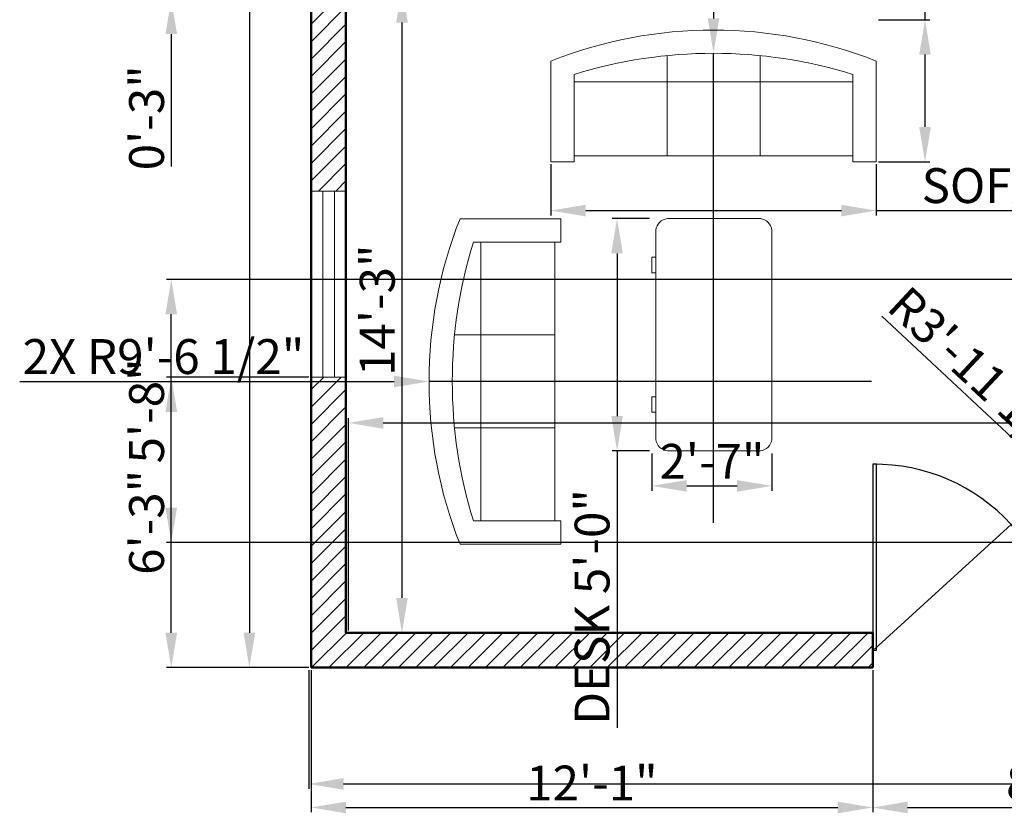
# Model space of a CAD drawing. Units: inches. Extents: x 61993 to 62774, y 55335 to 55871.
# Tile 1 of 6: x 61993 to 62247, y 55358 to 55563. Entities that reach past the tile are written whole.
import ezdxf

# ---------------------------------------------------------------- set-up
doc = ezdxf.new("R2010")
doc.units = ezdxf.units.IN
for name, color, linetype, lineweight in [('A-ANNO-DIMS', 2, 'Continuous', 18), ('A-DOOR', 3, 'Continuous', 25), ('A-FURN', 9, 'Continuous', 18), ('A-GLAZ', 4, 'Continuous', 18), ('A-WALL', 7, 'Continuous', 50)]:
    doc.layers.add(name, color=color, linetype=linetype, lineweight=lineweight)
doc.layers.add('A-WALL-PATT', color=40, linetype='Continuous', lineweight=13, true_color=0xf8d731)
doc.styles.get("Standard").update_dxf_attribs({"font": 'arial.ttf'})
doc.dimstyles.new('ISO-25', dxfattribs={"dimtxt": 9, "dimasz": 9, "dimexe": 1.25, "dimexo": 0.625, "dimtad": 1, "dimdec": 1, "dimrnd": 9, "dimlunit": 3, "dimtxsty": 'Standard', "dimcen": 2.5, "dimadec": 0, "dimazin": 0, "dimtfac": 1, "dimtdec": 1, "dimtmove": 0, "dimatfit": 3, "dimfxl": 1, "dimarcsym": 0})

# ---------------------------------------------------------------- blocks, each defined once
blk = doc.blocks.new('*D11')
at = {"layer": 'A-ANNO-DIMS', "color": 0, "lineweight": -2, "transparency": 16777216}
for p, q in [((62077.82, 55571.46), (62092.9, 55571.46)), ((62091.65, 55562.46), (62091.65, 55413.96)), ((62077.82, 55404.96), (62092.9, 55404.96))]:
    blk.add_line(p, q, dxfattribs=at)
at = {"layer": 'A-ANNO-DIMS', "color": 0, "transparency": 16777216}
for points in [[(62090.15, 55562.46), (62093.15, 55562.46), (62091.65, 55571.46)], [(62090.15, 55413.96), (62093.15, 55413.96), (62091.65, 55404.96)]]:
    blk.add_solid(points, dxfattribs=at)
at = {"layer": 'Defpoints', "color": 0, "transparency": 16777216}
for p in [(62077.19, 55571.46), (62077.19, 55404.96), (62091.65, 55404.96)]:
    blk.add_point(p, dxfattribs=at)
at = {"layer": 'A-ANNO-DIMS', "color": 0, "transparency": 16777216, "insert": (62086.43, 55488.21), "char_height": 9, "attachment_point": 5, "rotation": 90}
blk.add_mtext('14\'-3"', dxfattribs=at)
blk = doc.blocks.new('*D12')
at = {"layer": 'A-ANNO-DIMS', "color": 0, "lineweight": -2, "transparency": 16777216}
for p, q in [((62077.82, 55405.58), (62077.82, 55460.37)), ((62086.82, 55459.12), (62534.69, 55459.12)), ((62543.69, 55405.58), (62543.69, 55460.37))]:
    blk.add_line(p, q, dxfattribs=at)
at = {"layer": 'A-ANNO-DIMS', "color": 0, "transparency": 16777216}
for points in [[(62086.82, 55460.62), (62086.82, 55457.62), (62077.82, 55459.12)], [(62534.69, 55460.62), (62534.69, 55457.62), (62543.69, 55459.12)]]:
    blk.add_solid(points, dxfattribs=at)
at = {"layer": 'Defpoints', "color": 0, "transparency": 16777216}
for p in [(62543.69, 55459.12), (62077.82, 55404.96), (62543.69, 55404.96)]:
    blk.add_point(p, dxfattribs=at)
at = {"layer": 'A-ANNO-DIMS', "color": 0, "transparency": 16777216, "insert": (62310.76, 55464.35), "char_height": 9, "attachment_point": 5}
blk.add_mtext("39'", dxfattribs=at)
blk = doc.blocks.new('Sofa - Roundback 7 ft.')
for p, q in [((-12.00002, -32.4421), (-12.00003, -6.5971)), ((11.99997, -32.4421), (11.99998, -6.5971)), ((-36.000027, -34), (-36.000027, -11.4696)), ((35.99998, -34), (35.99998, -11.4696)), ((-35.999844, -13.3819), (35.9998, -13.3819)), ((-36.000027, -32.4421), (35.99998, -32.4421))]:
    blk.add_line(p, q)
for points in [[(-36.000027, -34), (-42.000027, -34), (-42.000027, -8)], [(41.99998, -8), (41.99998, -34), (35.99998, -34)]]:
    blk.add_lwpolyline(points)
for centre, radius, start, end in [((0, -114.25), 114.25, 68.43141, 111.5686), ((-0.00001, -127.1968), 121.1968, 72.72033, 107.2797)]:
    blk.add_arc(centre, radius, start, end)
blk = doc.blocks.new('Desk - 30 x 60 in.')
for p, q in [((-26.999995, 0), (26.999995, 0)), ((-29.999995, -27), (-29.999995, -3)), ((29.999995, -3), (29.999995, -27)), ((26.999995, -30), (-26.999995, -30)), ((-20.000005, -30), (-20.000005, -31)), ((-16.000005, -31), (-16.000005, -30)), ((15.999995, -31), (15.999995, -30)), ((19.999995, -30), (19.999995, -31)), ((-20.000005, -31), (-16.000005, -31)), ((19.999995, -31), (15.999995, -31))]:
    blk.add_line(p, q)
for centre, start, end in [((-26.499995, -3.5), 98.1301, 171.8699), ((26.499995, -3.5), 8.130102, 81.8699), ((-26.499995, -26.5), 188.1301, 261.8699), ((26.499995, -26.5), 278.1301, 351.8699)]:
    blk.add_arc(centre, 3.535534, start, end)
blk = doc.blocks.new('*D27')
at = {"layer": 'A-ANNO-DIMS', "color": 0, "lineweight": -2, "transparency": 16777216}
for p, q in [((62067.57, 55815.96), (62051, 55815.96)), ((62052.25, 55806.96), (62052.25, 55404.96)), ((62067.57, 55395.96), (62051, 55395.96))]:
    blk.add_line(p, q, dxfattribs=at)
at = {"layer": 'A-ANNO-DIMS', "color": 0, "transparency": 16777216}
for points in [[(62050.75, 55806.96), (62053.75, 55806.96), (62052.25, 55815.96)], [(62050.75, 55404.96), (62053.75, 55404.96), (62052.25, 55395.96)]]:
    blk.add_solid(points, dxfattribs=at)
at = {"layer": 'Defpoints', "color": 0, "transparency": 16777216}
for p in [(62068.19, 55815.96), (62052.25, 55395.96), (62068.19, 55395.96)]:
    blk.add_point(p, dxfattribs=at)
at = {"layer": 'A-ANNO-DIMS', "color": 0, "transparency": 16777216, "insert": (62047.03, 55605.96), "char_height": 9, "attachment_point": 5, "rotation": 90}
blk.add_mtext('35\'-3"', dxfattribs=at)
blk = doc.blocks.new('*D28')
at = {"layer": 'A-ANNO-DIMS', "color": 0, "lineweight": -2, "transparency": 16777216}
for p, q in [((62067.57, 55395.33), (62067.57, 55364.68)), ((62728.19, 55395.33), (62728.19, 55364.68)), ((62076.57, 55365.93), (62719.19, 55365.93))]:
    blk.add_line(p, q, dxfattribs=at)
at = {"layer": 'A-ANNO-DIMS', "color": 0, "transparency": 16777216}
for points in [[(62076.57, 55367.43), (62076.57, 55364.43), (62067.57, 55365.93)], [(62719.19, 55367.43), (62719.19, 55364.43), (62728.19, 55365.93)]]:
    blk.add_solid(points, dxfattribs=at)
at = {"layer": 'Defpoints', "color": 0, "transparency": 16777216}
for p in [(62067.57, 55395.96), (62728.19, 55395.96), (62728.19, 55365.93)]:
    blk.add_point(p, dxfattribs=at)
at = {"layer": 'A-ANNO-DIMS', "color": 0, "transparency": 16777216, "insert": (62397.88, 55371.15), "char_height": 9, "attachment_point": 5}
blk.add_mtext('54\'-9"', dxfattribs=at)
blk = doc.blocks.new('WIN-48IN')
for p, q in [((0, 9), (0, 0)), ((48, 9), (48, 0)), ((48, 6), (0, 6)), ((48, 3), (0, 3))]:
    blk.add_line(p, q)
blk = doc.blocks.new('*D42')
at = {"layer": 'A-ANNO-DIMS', "color": 0, "lineweight": -2, "transparency": 16777216}
for p, q in [((62130.08, 55525.89), (62130.08, 55512.67)), ((62214.08, 55525.89), (62214.08, 55512.67)), ((62139.08, 55513.92), (62205.08, 55513.92)), ((62214.08, 55513.92), (62316.87, 55513.92))]:
    blk.add_line(p, q, dxfattribs=at)
at = {"layer": 'A-ANNO-DIMS', "color": 0, "transparency": 16777216}
for points in [[(62139.08, 55515.42), (62139.08, 55512.42), (62130.08, 55513.92)], [(62205.08, 55515.42), (62205.08, 55512.42), (62214.08, 55513.92)]]:
    blk.add_solid(points, dxfattribs=at)
at = {"layer": 'Defpoints', "color": 0, "transparency": 16777216}
for p in [(62130.08, 55526.52), (62214.08, 55526.52), (62214.08, 55513.92)]:
    blk.add_point(p, dxfattribs=at)
at = {"layer": 'A-ANNO-DIMS', "color": 0, "transparency": 16777216, "insert": (62269.98, 55519.2), "char_height": 9, "attachment_point": 5}
blk.add_mtext('SOFA 7\'-0" TYP.', dxfattribs=at)
blk = doc.blocks.new('*D43')
at = {"layer": 'A-ANNO-DIMS', "color": 0, "lineweight": -2, "transparency": 16777216}
for p, q in [((62226.68, 55563.18), (62226.68, 55649.26)), ((62214.71, 55563.18), (62227.93, 55563.18)), ((62226.68, 55535.52), (62226.68, 55554.18)), ((62214.71, 55526.52), (62227.93, 55526.52))]:
    blk.add_line(p, q, dxfattribs=at)
at = {"layer": 'A-ANNO-DIMS', "color": 0, "transparency": 16777216}
for points in [[(62225.18, 55554.18), (62228.18, 55554.18), (62226.68, 55563.18)], [(62225.18, 55535.52), (62228.18, 55535.52), (62226.68, 55526.52)]]:
    blk.add_solid(points, dxfattribs=at)
at = {"layer": 'Defpoints', "color": 0, "transparency": 16777216}
for p in [(62214.08, 55563.18), (62226.68, 55563.18), (62214.08, 55526.52)]:
    blk.add_point(p, dxfattribs=at)
at = {"layer": 'A-ANNO-DIMS', "color": 0, "transparency": 16777216, "insert": (62221.4, 55610.72), "char_height": 9, "attachment_point": 5, "rotation": 90}
blk.add_mtext('3\'-0 1/2" TYP.', dxfattribs=at)
blk = doc.blocks.new('*D56')
at = {"layer": 'A-ANNO-DIMS', "color": 0, "lineweight": -2, "transparency": 16777216}
for p, q in [((62155.55, 55511.87), (62145.92, 55511.87)), ((62147.17, 55502.87), (62147.17, 55460.87)), ((62155.55, 55451.87), (62145.92, 55451.87)), ((62147.17, 55451.87), (62147.17, 55380.42))]:
    blk.add_line(p, q, dxfattribs=at)
at = {"layer": 'A-ANNO-DIMS', "color": 0, "transparency": 16777216}
for points in [[(62145.67, 55502.87), (62148.67, 55502.87), (62147.17, 55511.87)], [(62145.67, 55460.87), (62148.67, 55460.87), (62147.17, 55451.87)]]:
    blk.add_solid(points, dxfattribs=at)
at = {"layer": 'Defpoints', "color": 0, "transparency": 16777216}
for p in [(62156.17, 55511.87), (62147.17, 55451.87), (62156.17, 55451.87)]:
    blk.add_point(p, dxfattribs=at)
at = {"layer": 'A-ANNO-DIMS', "color": 0, "transparency": 16777216, "insert": (62141.89, 55411.64), "char_height": 9, "attachment_point": 5, "rotation": 90}
blk.add_mtext('DESK 5\'-0"', dxfattribs=at)
blk = doc.blocks.new('*D57')
at = {"layer": 'A-ANNO-DIMS', "color": 0, "lineweight": -2, "transparency": 16777216}
for p, q in [((62156.17, 55451.25), (62156.17, 55441.62)), ((62187.17, 55451.25), (62187.17, 55441.62)), ((62165.17, 55442.87), (62178.17, 55442.87))]:
    blk.add_line(p, q, dxfattribs=at)
at = {"layer": 'A-ANNO-DIMS', "color": 0, "transparency": 16777216}
for points in [[(62165.17, 55444.37), (62165.17, 55441.37), (62156.17, 55442.87)], [(62178.17, 55444.37), (62178.17, 55441.37), (62187.17, 55442.87)]]:
    blk.add_solid(points, dxfattribs=at)
at = {"layer": 'Defpoints', "color": 0, "transparency": 16777216}
for p in [(62156.17, 55451.87), (62187.17, 55451.87), (62187.17, 55442.87)]:
    blk.add_point(p, dxfattribs=at)
at = {"layer": 'A-ANNO-DIMS', "color": 0, "transparency": 16777216, "insert": (62171.67, 55448.02), "char_height": 9, "attachment_point": 5}
blk.add_mtext('2\'-7"', dxfattribs=at)
blk = doc.blocks.new('*D60')
at = {"layer": 'A-ANNO-DIMS', "color": 0, "lineweight": -2, "transparency": 16777216}
for p, q in [((62213.17, 55395.33), (62213.17, 55358.61)), ((62309.17, 55395.33), (62309.17, 55358.61)), ((62222.17, 55359.86), (62300.17, 55359.86))]:
    blk.add_line(p, q, dxfattribs=at)
at = {"layer": 'A-ANNO-DIMS', "color": 0, "transparency": 16777216}
for points in [[(62222.17, 55361.36), (62222.17, 55358.36), (62213.17, 55359.86)], [(62300.17, 55361.36), (62300.17, 55358.36), (62309.17, 55359.86)]]:
    blk.add_solid(points, dxfattribs=at)
at = {"layer": 'Defpoints', "color": 0, "transparency": 16777216}
for p in [(62213.17, 55395.96), (62309.17, 55395.96), (62309.17, 55359.86)]:
    blk.add_point(p, dxfattribs=at)
at = {"layer": 'A-ANNO-DIMS', "color": 0, "transparency": 16777216, "insert": (62261.17, 55365.08), "char_height": 9, "attachment_point": 5}
blk.add_mtext('8\'-0"', dxfattribs=at)
blk = doc.blocks.new('*D61')
at = {"layer": 'A-ANNO-DIMS', "color": 0, "lineweight": -2, "transparency": 16777216}
for p, q in [((62068.19, 55395.33), (62068.19, 55358.61)), ((62213.17, 55395.33), (62213.17, 55358.61)), ((62077.19, 55359.86), (62204.17, 55359.86))]:
    blk.add_line(p, q, dxfattribs=at)
at = {"layer": 'A-ANNO-DIMS', "color": 0, "transparency": 16777216}
for points in [[(62077.19, 55361.36), (62077.19, 55358.36), (62068.19, 55359.86)], [(62204.17, 55361.36), (62204.17, 55358.36), (62213.17, 55359.86)]]:
    blk.add_solid(points, dxfattribs=at)
at = {"layer": 'Defpoints', "color": 0, "transparency": 16777216}
for p in [(62068.19, 55395.96), (62213.17, 55395.96), (62213.17, 55359.86)]:
    blk.add_point(p, dxfattribs=at)
at = {"layer": 'A-ANNO-DIMS', "color": 0, "transparency": 16777216, "insert": (62140.68, 55365), "char_height": 9, "attachment_point": 5}
blk.add_mtext('12\'-1"', dxfattribs=at)
blk = doc.blocks.new('*D68')
at = {"layer": 'A-ANNO-DIMS', "color": 0, "lineweight": -2, "transparency": 16777216}
for p, q in [((62067.57, 55470.96), (62030.84, 55470.96)), ((62032.09, 55404.96), (62032.09, 55461.96)), ((62067.57, 55395.96), (62030.84, 55395.96))]:
    blk.add_line(p, q, dxfattribs=at)
at = {"layer": 'A-ANNO-DIMS', "color": 0, "transparency": 16777216}
for points in [[(62030.59, 55461.96), (62033.59, 55461.96), (62032.09, 55470.96)], [(62030.59, 55404.96), (62033.59, 55404.96), (62032.09, 55395.96)]]:
    blk.add_solid(points, dxfattribs=at)
at = {"layer": 'Defpoints', "color": 0, "transparency": 16777216}
for p in [(62032.09, 55470.96), (62068.19, 55470.96), (62068.19, 55395.96)]:
    blk.add_point(p, dxfattribs=at)
at = {"layer": 'A-ANNO-DIMS', "color": 0, "transparency": 16777216, "insert": (62026.87, 55433.46), "char_height": 9, "attachment_point": 5, "rotation": 90}
blk.add_mtext('6\'-3"', dxfattribs=at)
blk = doc.blocks.new('*D74')
at = {"layer": 'A-ANNO-DIMS', "color": 0, "lineweight": -2, "transparency": 16777216}
for p, q in [((62032.09, 55580.46), (62032.09, 55589.46)), ((62547.57, 55571.46), (62030.84, 55571.46)), ((62032.09, 55571.46), (62032.09, 55568.46)), ((62547.57, 55568.46), (62030.84, 55568.46)), ((62032.09, 55559.46), (62032.09, 55525.28))]:
    blk.add_line(p, q, dxfattribs=at)
at = {"layer": 'A-ANNO-DIMS', "color": 0, "transparency": 16777216}
for points in [[(62030.59, 55580.46), (62033.59, 55580.46), (62032.09, 55571.46)], [(62030.59, 55559.46), (62033.59, 55559.46), (62032.09, 55568.46)]]:
    blk.add_solid(points, dxfattribs=at)
at = {"layer": 'Defpoints', "color": 0, "transparency": 16777216}
for p in [(62548.19, 55571.46), (62032.09, 55568.46), (62548.19, 55568.46)]:
    blk.add_point(p, dxfattribs=at)
at = {"layer": 'A-ANNO-DIMS', "color": 0, "transparency": 16777216, "insert": (62026.87, 55537.87), "char_height": 9, "attachment_point": 5, "rotation": 90}
blk.add_mtext('0\'-3"', dxfattribs=at)
blk = doc.blocks.new('*D80')
at = {"layer": 'A-ANNO-DIMS', "color": 0, "lineweight": -2, "transparency": 16777216}
for p, q in [((62558.29, 55496.17), (62030.84, 55496.17)), ((62032.09, 55437.26), (62032.09, 55487.17)), ((62558.29, 55428.26), (62030.84, 55428.26))]:
    blk.add_line(p, q, dxfattribs=at)
at = {"layer": 'A-ANNO-DIMS', "color": 0, "transparency": 16777216}
for points in [[(62030.59, 55487.17), (62033.59, 55487.17), (62032.09, 55496.17)], [(62030.59, 55437.26), (62033.59, 55437.26), (62032.09, 55428.26)]]:
    blk.add_solid(points, dxfattribs=at)
at = {"layer": 'Defpoints', "color": 0, "transparency": 16777216}
for p in [(62032.09, 55496.17), (62558.91, 55496.17), (62558.91, 55428.26)]:
    blk.add_point(p, dxfattribs=at)
at = {"layer": 'A-ANNO-DIMS', "color": 0, "transparency": 16777216, "insert": (62026.87, 55462.22), "char_height": 9, "attachment_point": 5, "rotation": 90}
blk.add_mtext('5\'-8"', dxfattribs=at)
blk = doc.blocks.new('*D83')
at = {"layer": 'A-ANNO-DIMS', "color": 0, "lineweight": -2, "transparency": 16777216}
for p, q in [((62172.08, 55657.37), (62172.08, 55563.52)), ((62172.08, 55433.32), (62172.08, 55554.52))]:
    blk.add_line(p, q, dxfattribs=at)
at = {"layer": 'A-ANNO-DIMS', "color": 0, "transparency": 16777216}
blk.add_solid([(62173.58, 55563.52), (62170.58, 55563.52), (62172.08, 55554.52)], dxfattribs=at)
at = {"layer": 'Defpoints', "color": 0, "transparency": 16777216}
for p in [(62172.08, 55554.52), (62172.08, 55433.32)]:
    blk.add_point(p, dxfattribs=at)
at = {"layer": 'A-ANNO-DIMS', "color": 0, "transparency": 16777216, "insert": (62177.3, 55627.24), "char_height": 9, "attachment_point": 5, "rotation": 270.0001}
blk.add_mtext('2X R10\'-1"', dxfattribs=at)
blk = doc.blocks.new('*D84')
at = {"layer": 'A-ANNO-DIMS', "color": 0, "lineweight": -2, "transparency": 16777216}
for p, q in [((61992.96, 55469.81), (62089.63, 55469.81)), ((62212.88, 55469.81), (62098.63, 55469.81))]:
    blk.add_line(p, q, dxfattribs=at)
at = {"layer": 'A-ANNO-DIMS', "color": 0, "transparency": 16777216}
blk.add_solid([(62089.63, 55471.31), (62089.63, 55468.31), (62098.63, 55469.81)], dxfattribs=at)
at = {"layer": 'Defpoints', "color": 0, "transparency": 16777216}
for p in [(62098.63, 55469.81), (62212.88, 55469.81)]:
    blk.add_point(p, dxfattribs=at)
at = {"layer": 'A-ANNO-DIMS', "color": 0, "transparency": 16777216, "insert": (62030.08, 55475.08), "char_height": 9, "attachment_point": 5, "rotation": 359.9999}
blk.add_mtext('2X R9\'-6 1/2"', dxfattribs=at)
blk = doc.blocks.new('*D85')
at = {"layer": 'A-ANNO-DIMS', "color": 0, "lineweight": -2, "transparency": 16777216}
for p, q in [((62307.76, 55486.75), (62255.54, 55439.01)), ((62213.67, 55400.72), (62248.9, 55432.93))]:
    blk.add_line(p, q, dxfattribs=at)
at = {"layer": 'A-ANNO-DIMS', "color": 0, "transparency": 16777216}
blk.add_solid([(62254.53, 55440.11), (62256.56, 55437.9), (62248.9, 55432.93)], dxfattribs=at)
at = {"layer": 'Defpoints', "color": 0, "transparency": 16777216}
for p in [(62248.9, 55432.93), (62213.67, 55400.72)]:
    blk.add_point(p, dxfattribs=at)
at = {"layer": 'A-ANNO-DIMS', "color": 0, "transparency": 16777216, "insert": (62281.41, 55469.81), "char_height": 9, "attachment_point": 5, "rotation": 42.4359}
blk.add_mtext('R3\'-11 1/2"', dxfattribs=at)
blk = doc.blocks.new('*D86')
at = {"layer": 'A-ANNO-DIMS', "color": 0, "lineweight": -2, "transparency": 16777216}
for p, q in [((62215.49, 55486.67), (62267.24, 55438.41)), ((62308.67, 55399.78), (62273.82, 55432.28))]:
    blk.add_line(p, q, dxfattribs=at)
at = {"layer": 'A-ANNO-DIMS', "color": 0, "transparency": 16777216}
blk.add_solid([(62268.26, 55439.51), (62266.21, 55437.32), (62273.82, 55432.28)], dxfattribs=at)
at = {"layer": 'Defpoints', "color": 0, "transparency": 16777216}
for p in [(62273.82, 55432.28), (62308.67, 55399.78)]:
    blk.add_point(p, dxfattribs=at)
at = {"layer": 'A-ANNO-DIMS', "color": 0, "transparency": 16777216, "insert": (62241.68, 55469.47), "char_height": 9, "attachment_point": 5, "rotation": 316.998}
blk.add_mtext('R3\'-11 1/2"', dxfattribs=at)

msp = doc.modelspace()

# ---------------------------------------------------------------- hatches: boundary and pattern name
at = {"layer": 'A-WALL-PATT'}
h = msp.add_hatch(dxfattribs=at)
h.set_pattern_fill('ANSI31', color=256)
h.paths.add_polyline_path([(62077.19, 55665.16), (62068.19, 55665.16), (62068.19, 55518.96), (62077.19, 55518.96), (62077.19, 55571.46), (62234.23, 55571.46), (62234.23, 55573.71, -0.007042), (62234.23, 55574.71), (62234.23, 55575.96), (62077.19, 55575.96)])
h.paths.add_polyline_path([(62077.19, 55806.96), (62138.51, 55806.96), (62138.51, 55815.96), (62068.19, 55815.96), (62068.19, 55713.16), (62077.19, 55713.16)])
h.paths.add_polyline_path([(62364.31, 55815.96), (62186.51, 55815.96), (62186.51, 55806.96), (62308.19, 55806.96), (62308.19, 55575.96), (62270.23, 55575.96), (62270.23, 55571.46), (62415.32, 55571.46), (62415.32, 55573.71, -0.007042), (62415.32, 55574.71), (62415.32, 55575.96), (62312.69, 55575.96), (62312.69, 55739.46), (62471.69, 55739.46), (62471.69, 55575.96), (62451.32, 55575.96), (62451.32, 55571.46), (62483.74, 55571.46), (62483.74, 55573.71, -0.007042), (62483.74, 55574.71), (62483.74, 55575.96), (62476.19, 55575.96), (62476.19, 55806.96), (62578.07, 55806.96), (62578.07, 55815.96), (62412.31, 55815.96), (62412.31, 55806.96), (62471.69, 55806.96), (62471.69, 55743.96), (62312.69, 55743.96), (62312.69, 55806.96), (62364.31, 55806.96)])
h.paths.add_polyline_path([(62728.19, 55815.96), (62626.07, 55815.96), (62626.07, 55806.96), (62719.19, 55806.96), (62719.19, 55739.46), (62728.19, 55739.46)])
h.paths.add_polyline_path([(62728.19, 55691.46), (62719.19, 55691.46), (62719.19, 55575.96), (62519.74, 55575.96), (62519.74, 55571.46), (62543.69, 55571.46), (62543.69, 55568.46), (62548.19, 55568.46), (62548.19, 55571.46), (62719.19, 55571.46), (62719.19, 55517.72), (62728.19, 55517.72)])
h.paths.add_polyline_path([(62599.31, 55404.96), (62548.19, 55404.96), (62548.19, 55532.46), (62546.94, 55532.46, -0.007042), (62545.94, 55532.46), (62543.69, 55532.46), (62543.69, 55404.96), (62444.22, 55404.96), (62444.22, 55395.96), (62599.31, 55395.96)])
h.paths.add_polyline_path([(62728.19, 55469.72), (62719.19, 55469.72), (62719.19, 55404.96), (62647.31, 55404.96), (62647.31, 55395.96), (62728.19, 55395.96)])
h.paths.add_polyline_path([(62396.22, 55404.96), (62309.17, 55404.96), (62309.17, 55395.96), (62396.22, 55395.96)])
h.paths.add_polyline_path([(62213.17, 55404.96), (62077.19, 55404.96), (62077.19, 55470.96), (62068.19, 55470.96), (62068.19, 55395.96), (62213.17, 55395.96)])

# ---------------------------------------------------------------- linework, layer by layer
at = {"layer": 'A-DOOR'}
for p, q in [((62214.17, 55448.46), (62213.17, 55448.46)), ((62213.17, 55448.46), (62213.17, 55404.96)), ((62214.17, 55400.46), (62214.17, 55448.46)), ((62213.17, 55400.46), (62214.17, 55400.46))]:
    msp.add_line(p, q, dxfattribs=at)
msp.add_arc((62213.67, 55400.72), 47.74, 354.2723, 90.6001, dxfattribs=at)
at = {"layer": 'A-WALL'}
for p, q in [((62068.19, 55815.96), (62068.19, 55395.96)), ((62077.19, 55571.46), (62077.19, 55404.96)), ((62077.19, 55404.96), (62213.17, 55404.96)), ((62213.17, 55404.96), (62213.17, 55395.96)), ((62068.19, 55395.96), (62213.17, 55395.96))]:
    msp.add_line(p, q, dxfattribs=at)

# ---------------------------------------------------------------- block references
at = {"layer": 'A-FURN'}
msp.add_blockref('Sofa - Roundback 7 ft.', (62172.08, 55560.52), dxfattribs=at)
for name, p, rotation in [('Sofa - Roundback 7 ft.', (62098.63, 55469.81), 90), ('Desk - 30 x 60 in.', (62187.17, 55481.87), 270)]:
    msp.add_blockref(name, p, dxfattribs=dict(at, rotation=rotation))
at = {"layer": 'A-GLAZ', "rotation": 269.9999999999937}
msp.add_blockref('WIN-48IN', (62068.19, 55518.96), dxfattribs=at)

# ---------------------------------------------------------------- dimensions: what is measured, and where the dimension line sits
at = {"layer": 'A-ANNO-DIMS'}
for base, p1, p2, override, picture, middle in [((62052.25, 55395.96), (62068.19, 55815.96), (62068.19, 55395.96), {"dimclrd": 0, "dimclre": 0, "dimclrt": 0}, '*D27', (62047.03, 55605.96)), ((62032.09, 55568.46), (62548.19, 55571.46), (62548.19, 55568.46), {"dimdec": 1, "dimlfac": 1, "dimrnd": 0, "dimzin": 1, "dimdsep": 46, "dimlunit": 4, "dimfrac": 2}, '*D74', (62026.87, 55537.87)), ((62091.65, 55404.96), (62077.19, 55571.46), (62077.19, 55404.96), {"dimclrd": 0, "dimclre": 0, "dimclrt": 0}, '*D11', (62086.43, 55488.21)), ((62032.09, 55496.17), (62558.91, 55428.26), (62558.91, 55496.17), {"dimdec": 1, "dimlfac": 1, "dimrnd": 0, "dimzin": 1, "dimdsep": 46, "dimlunit": 4, "dimfrac": 2}, '*D80', (62026.87, 55462.22)), ((62032.09, 55470.96), (62068.19, 55395.96), (62068.19, 55470.96), {"dimdec": 1, "dimlfac": 1, "dimrnd": 0, "dimzin": 1, "dimdsep": 46, "dimlunit": 4, "dimfrac": 2}, '*D68', (62026.87, 55433.46))]:
    dim = msp.add_linear_dim(base=base, p1=p1, p2=p2, angle=90, dimstyle='ISO-25', override=override, dxfattribs=at)
    dim.commit()
    dim.dimension.update_dxf_attribs({"geometry": picture, "text_midpoint": middle})
for center, mpoint, picture, middle in [((62172.08, 55433.32), (62172.08, 55554.52), '*D83', (62172.08, 55627.24)), ((62212.883919, 55469.805834), (62098.633919, 55469.806), '*D84', (62030.083919, 55469.8060996))]:
    dim = msp.add_radius_dim(center=center, mpoint=mpoint, text='2X <>', dimstyle='ISO-25', override={"dimdec": 1, "dimlfac": 1, "dimrnd": 0, "dimzin": 1, "dimdsep": 46, "dimlunit": 4, "dimfrac": 2}, dxfattribs=at)
    dim.commit()
    dim.dimension.update_dxf_attribs({"geometry": picture, "text_midpoint": middle, "dimtype": 164})
for base, p1, p2, angle, text, picture, middle in [((62226.68, 55563.18), (62214.08, 55526.52), (62214.08, 55563.18), 90, '<> TYP.', '*D43', (62221.4, 55610.72)), ((62147.17, 55451.87), (62156.17, 55511.87), (62156.17, 55451.87), 270, 'DESK <>', '*D56', (62141.89, 55411.64))]:
    dim = msp.add_linear_dim(base=base, p1=p1, p2=p2, angle=angle, text=text, dimstyle='ISO-25', override={"dimdec": 1, "dimlfac": 1, "dimrnd": 0, "dimzin": 1, "dimdsep": 46, "dimlunit": 4, "dimfrac": 2}, dxfattribs=at)
    dim.commit()
    dim.dimension.update_dxf_attribs({"geometry": picture, "text_midpoint": middle})
dim = msp.add_linear_dim(base=(62214.08, 55513.92), p1=(62130.08, 55526.52), p2=(62214.08, 55526.52), text='SOFA <> TYP.', dimstyle='ISO-25', override={"dimdec": 1, "dimlfac": 1, "dimrnd": 0, "dimzin": 1, "dimdsep": 46, "dimlunit": 4, "dimfrac": 2}, dxfattribs=at)
dim.commit()
dim.dimension.update_dxf_attribs({"geometry": '*D42', "text_midpoint": (62269.98, 55519.2)})
for center, mpoint, picture, middle in [((62213.67, 55400.72), (62248.9, 55432.93), '*D85', (62281.41, 55469.81)), ((62308.67, 55399.78), (62273.82, 55432.28), '*D86', (62241.68, 55469.47))]:
    dim = msp.add_radius_dim(center=center, mpoint=mpoint, dimstyle='ISO-25', override={"dimdec": 1, "dimlfac": 1, "dimrnd": 0, "dimzin": 1, "dimdsep": 46, "dimlunit": 4, "dimfrac": 2}, dxfattribs=at)
    dim.commit()
    dim.dimension.update_dxf_attribs({"geometry": picture, "text_midpoint": middle})
for base, p1, p2, override, picture, middle in [((62543.69, 55459.12), (62077.82, 55404.96), (62543.69, 55404.96), {"dimclrd": 0, "dimclre": 0, "dimclrt": 0}, '*D12', (62310.76, 55464.35)), ((62187.17, 55442.87), (62156.17, 55451.87), (62187.17, 55451.87), {"dimdec": 1, "dimlfac": 1, "dimrnd": 0, "dimzin": 1, "dimdsep": 46, "dimlunit": 4, "dimfrac": 2}, '*D57', (62171.67, 55448.02)), ((62213.17, 55359.86), (62068.19, 55395.96), (62213.17, 55395.96), {"dimdec": 1, "dimlfac": 1, "dimrnd": 0, "dimzin": 1, "dimdsep": 46, "dimlunit": 4, "dimfrac": 2}, '*D61', (62140.68, 55365)), ((62309.17, 55359.86), (62213.17, 55395.96), (62309.17, 55395.96), {"dimdec": 1, "dimlfac": 1, "dimrnd": 0, "dimzin": 1, "dimdsep": 46, "dimlunit": 4, "dimfrac": 2}, '*D60', (62261.17, 55365.08))]:
    dim = msp.add_linear_dim(base=base, p1=p1, p2=p2, dimstyle='ISO-25', override=override, dxfattribs=at)
    dim.commit()
    dim.dimension.update_dxf_attribs({"geometry": picture, "text_midpoint": middle})
dim = msp.add_aligned_dim(p1=(62067.57, 55395.96), p2=(62728.19, 55395.96), distance=-30.03, dimstyle='ISO-25', override={"dimclrd": 0, "dimclre": 0, "dimclrt": 0}, dxfattribs=at)
dim.commit()
dim.dimension.update_dxf_attribs({"geometry": '*D28', "text_midpoint": (62397.88, 55371.15)})

doc.saveas('drawing.dxf')
